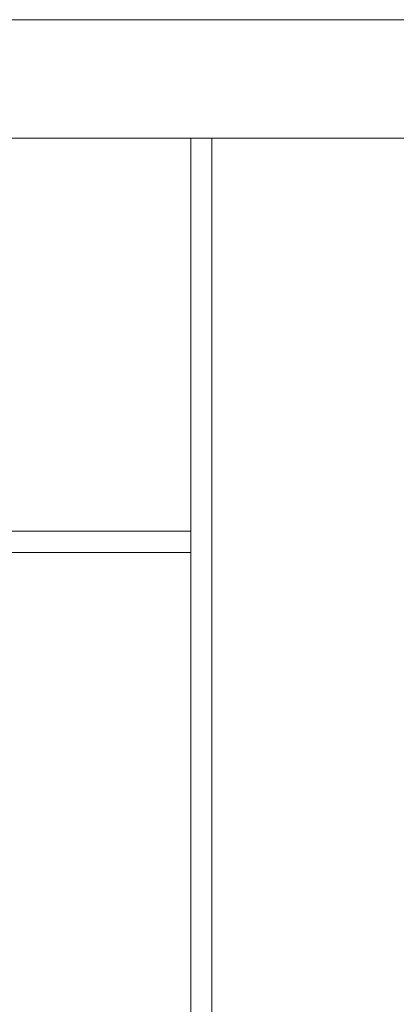
# Model space of a CAD drawing. Units: inches. Extents: x -17 to 1735, y -531 to 60.
# Tile 14 of 27: x 1734.68152 to 1734.69407, y -150.19886 to -150.16612. Entities that reach past the tile are written whole.
import ezdxf

# ---------------------------------------------------------------- set-up
doc = ezdxf.new("R2010")
doc.units = ezdxf.units.IN
doc.header["$MEASUREMENT"] = 0
doc.layers.add('A-FURN', color=242, linetype='Continuous', lineweight=18, true_color=0xcd2027)

# ---------------------------------------------------------------- blocks, each defined once
blk = doc.blocks.new('childrens_room_2')
for p, q in [((69.73591, 55.43419), (71.79591, 55.43419)), ((69.75691, 55.33419), (71.77791, 55.33419)), ((70.47533, 55.33419), (70.47533, 53.9594)), ((70.49333, 55.33419), (70.49333, 53.9594)), ((69.75691, 55.00219), (70.47533, 55.00219)), ((69.75691, 54.98419), (70.47533, 54.98419))]:
    blk.add_line(p, q)

msp = doc.modelspace()

# ---------------------------------------------------------------- block references
at = {"layer": 'A-FURN', "xscale": 0.0393700787401575, "yscale": 0.0393700787401575, "zscale": 0.0393700787401575}
msp.add_blockref('childrens_room_2', (1731.912601, -152.348565), dxfattribs=at)

doc.saveas('drawing.dxf')
